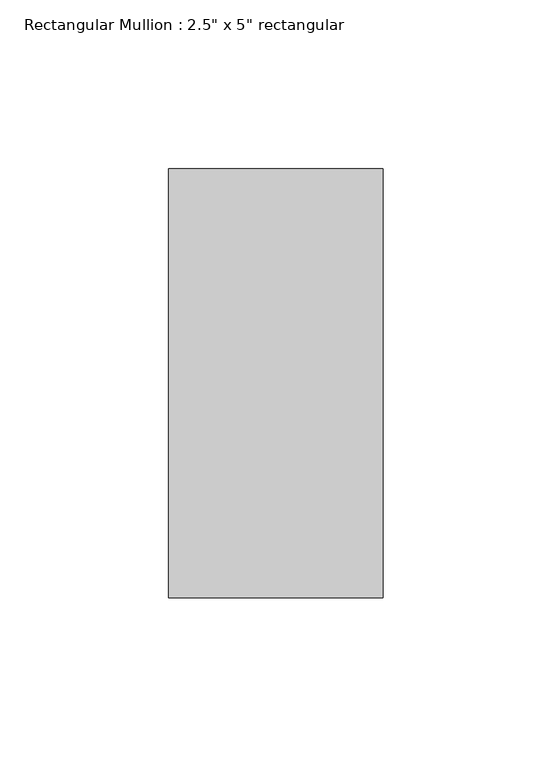
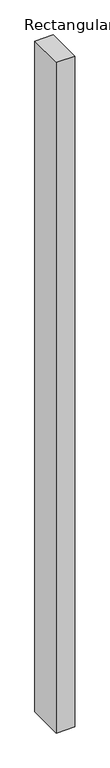
"""IFC4 building model written with IfcOpenShell, lengths in millimetres: member geometry."""

from ifc_helpers import new_model, si_unit, frame, origin, place, context, project, spatial, polyline, outline, extrude, source, transform, mapped, element, save


def member_f0fea5a5(model_context):
    return source(origin(), model_context, "Body", "SweptSolid", [
        extrude(outline(polyline([(31.75, 63.5), (31.75, -63.5), (-31.75, -63.5), (-31.75, 63.5), (31.75, 63.5)])), frame((0.0, 0.0, -2438.4), z_axis=(0.0, 0.0, 1.0), x_axis=(1.0, 0.0, 0.0)), (0.0, 0.0, 1.0), 2438.4),
    ])


if __name__ == "__main__":
    model = new_model("IFC4")
    model_context = context("Model", 3, world=origin())
    ifc_project = project(units=[si_unit("LENGTHUNIT", "METRE", prefix="MILLI")], contexts=[model_context])
    site = spatial("IfcSite", under=ifc_project)
    building = spatial("IfcBuilding", under=site)
    placement = place(None, origin())
    member_shape = member_f0fea5a5(model_context)
    element("IfcMember", 1, ObjectType="Rectangular Mullion : 2.5\" x 5\" rectangular", at=placement, inside=building, context=model_context, shape_type="MappedRepresentation", body=[
        mapped(member_shape, transform((0.0, 0.0, 0.0), x_axis=(1.0, 0.0, 0.0), y_axis=(0.0, 1.0, 0.0), z_axis=(0.0, 0.0, 1.0))),
    ])
    save(model, "model.ifc")

# Revit data of these elements
# Type "Rectangular Mullion : 2.5\" x 5\" rectangular"
#   built-in parameter 1007304 = 0.416667 (stored number, unit not read)
#   built-in parameter 1007301 = 0.104167 (stored number, unit not read)
#   built-in parameter 1007300 = 0.104167 (stored number, unit not read)
# Element 1 (IfcMember, "Rectangular Mullion : 2.5\" x 5\" rectangular")
#   Materials on its faces: "mullions"
# Materials
#   "mullions": class "Generic", colour RGB 120 120 120, transparency 0, Cost = 0
